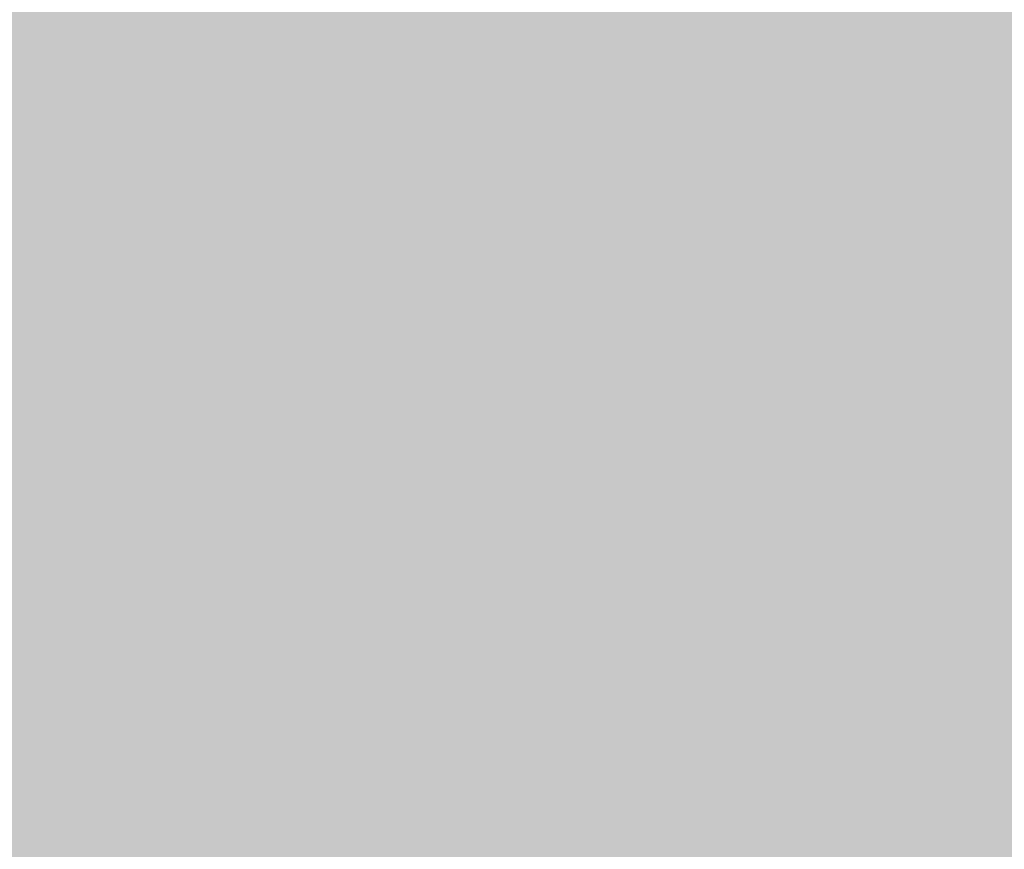
# Model space of a CAD drawing. Units: feet. Extents: x 3168 to 4724, y 827 to 1477.
# Tile 65 of 256: x 3273.15625 to 3273.17306, y 1099.00068 to 1099.01485. Entities that reach past the tile are written whole.
import ezdxf

# ---------------------------------------------------------------- set-up
doc = ezdxf.new("R2010")
doc.units = ezdxf.units.FT
doc.layers.add('A-ELEV', color=7, linetype='Continuous', lineweight=35)
doc.layers.add('A-ELEV-PATT', color=8, linetype='Continuous', lineweight=13)

msp = doc.modelspace()

# ---------------------------------------------------------------- hatches: boundary and pattern name
at = {"layer": 'A-ELEV-PATT'}
h = msp.add_hatch(color=256, dxfattribs=at)
h.dxf.hatch_style = 1
edge = h.paths.add_edge_path()
edge.add_ellipse((3552.905762, 979.220141), major_axis=(36.744924, 0), ratio=0.484848485, start_angle=0, end_angle=360)
edge = h.paths.add_edge_path()
edge.add_ellipse((3559.891637, 929.252282), major_axis=(36.744924, 0), ratio=0.484848485, start_angle=0, end_angle=360)
edge = h.paths.add_edge_path()
edge.add_line((3299.31681, 1198.606081), (3479.916714, 1198.606081))
edge.add_line((3479.916714, 1198.606081), (3479.916714, 1209.86857))
edge.add_spline(control_points=[(3479.916714, 1209.86857), (3464.301157, 1209.86857), (3448.685601, 1209.86857), (3410.949139, 1209.86857), (3388.828234, 1209.86857), (3355.646876, 1209.86857), (3344.586423, 1209.86857), (3327.995745, 1209.86857), (3322.465518, 1209.86857), (3314.170179, 1209.86857), (3311.405066, 1209.86857), (3307.257396, 1209.86857), (3305.874839, 1209.86857), (3303.801005, 1209.86857), (3303.109726, 1209.86857), (3302.072809, 1209.86857), (3301.72717, 1209.86857), (3301.208711, 1209.86857), (3301.035891, 1209.86857), (3300.776662, 1209.86857), (3300.690252, 1209.86857), (3300.560638, 1209.86857), (3300.517433, 1209.86857), (3300.452625, 1209.86857), (3300.431023, 1209.86857), (3300.398619, 1209.86857), (3300.387818, 1209.86857), (3300.366216, 1209.86857), (3300.345676, 1209.86857), (3300.345548, 1209.86857), (3300.345505, 1209.86857), (3300.343304, 1209.86857), (3300.341146, 1209.868571), (3300.337909, 1209.868571), (3300.33683, 1209.868572), (3300.333942, 1209.868573), (3300.332133, 1209.868574), (3300.325515, 1209.868577), (3300.320706, 1209.868581), (3300.310925, 1209.868592), (3300.305952, 1209.868598), (3300.290511, 1209.868623), (3300.280045, 1209.868646), (3300.232425, 1209.868777), (3300.195298, 1209.868954), (3299.951068, 1209.870608), (3299.744824, 1209.874326), (3299.436827, 1209.883257), (3299.334389, 1209.886792), (3299.181079, 1209.89292), (3299.130033, 1209.895099), (3298.652217, 1209.916801), (3298.22946, 1209.945718), (3297.601631, 1210.002367), (3297.393404, 1210.023464), (3297.082652, 1210.058309), (3296.979332, 1210.070458), (3296.292954, 1210.154861), (3295.718148, 1210.243356), (3294.868717, 1210.39885), (3294.5877, 1210.454478), (3294.169341, 1210.543349), (3294.030415, 1210.573878), (3291.707149, 1211.1012), (3289.65359, 1211.813435), (3285.776259, 1213.563988), (3283.95141, 1214.603478), (3280.512159, 1216.98008), (3278.897241, 1218.317592), (3276.379914, 1220.829489), (3275.416042, 1221.917738), (3274.039342, 1223.7077), (3273.581043, 1224.349535), (3273.143228, 1225.016316)], knot_values=[39.119033, 39.119033, 39.119033, 39.119033, 39.286353, 39.286353, 39.523379, 39.523379, 39.641892, 39.641892, 39.701148, 39.701148, 39.730777, 39.730777, 39.745591, 39.745591, 39.752998, 39.752998, 39.756701, 39.756701, 39.758553, 39.758553, 39.759479, 39.759479, 39.759942, 39.759942, 39.760173, 39.760173, 39.760289, 39.760289, 39.760405, 39.760405, 39.760463, 39.760463, 39.763389, 39.763389, 39.764851, 39.764851, 39.767304, 39.767304, 39.773825, 39.773825, 39.78057, 39.78057, 39.79477, 39.79477, 39.845194, 39.845194, 40.126715, 40.126715, 40.267476, 40.267476, 40.337856, 40.337856, 40.927023, 40.927023, 41.221606, 41.221606, 41.368898, 41.368898, 42.202622, 42.202622, 42.619485, 42.619485, 42.827916, 42.827916, 46.118323, 46.118323, 49.408731, 49.408731, 52.699139, 52.699139, 54.927489, 54.927489, 56.104228, 56.104228, 56.104228, 56.104228], weights=[1, 1, 1, 1, 1, 1, 1, 1, 1, 1, 1, 1, 1, 1, 1, 1, 1, 1, 1, 1, 1, 1, 1, 1, 1, 1, 1, 1, 1, 1, 1, 1, 1, 1, 1, 1, 1, 1, 1, 1, 1, 1, 1, 1, 1, 1, 1, 1, 1, 1, 1, 1, 1, 1, 1, 1, 1, 1, 1, 1, 1, 1, 1, 1, 1, 1, 1, 1, 1, 1, 1, 1, 1, 1], degree=3, periodic=0)
edge.add_line((3273.143228, 1225.016316), (3273.143228, 1099.016316))
edge.add_line((3273.143228, 1099.016316), (3299.31681, 1099.016316))
edge.add_line((3299.31681, 1099.016316), (3299.31681, 1198.606081))
edge = h.paths.add_edge_path()
edge.add_line((3304.758443, 1324.15806), (3479.916714, 1324.15806))
edge.add_line((3479.916714, 1324.15806), (3479.916714, 1335.714618))
edge.add_line((3479.916714, 1335.714618), (3269.161628, 1335.714618))
edge.add_spline(control_points=[(3269.161628, 1335.714618), (3264.024231, 1335.714618), (3258.364118, 1328.958189), (3259.264311, 1323.900274)], knot_values=[0, 0, 0, 0, 15.412191, 15.412191, 15.412191, 15.412191], degree=3, periodic=0)
edge.add_line((3259.264311, 1323.900274), (3265.516849, 1288.769135))
edge.add_line((3265.516849, 1288.769135), (3275.265103, 1261.545626))
edge.add_line((3275.265103, 1261.545626), (3304.758443, 1261.545626))
edge.add_line((3304.758443, 1261.545626), (3304.758443, 1324.15806))
h = msp.add_hatch(color=256, dxfattribs=at)
h.dxf.hatch_style = 1
h.paths.add_polyline_path([(3384.525247, 1099.016316), (3335.029168, 1099.016316), (3299.31681, 1099.016316), (3273.143228, 1099.016316), (3217.565364, 1099.016316), (3168.069285, 827.11626), (3335.029168, 827.11626)])

# ---------------------------------------------------------------- linework, layer by layer
at = {"layer": 'A-ELEV'}
msp.add_open_spline([(3808.5202, 1099.016316), (3808.5202, 1141.413235), (3808.5202, 1183.810154), (3808.5202, 1226.635324), (3808.5202, 1227.063576), (3808.5202, 1227.491828), (3811.491871, 1248.994673), (3814.463542, 1270.497518), (3817.46523, 1292.217564), (3817.495247, 1292.434764), (3817.525264, 1292.651964), (3817.572801, 1310.106748), (3817.620339, 1327.561532), (3817.667877, 1345.016316), (3817.667877, 1345.457962), (3817.667877, 1345.899608), (3817.667877, 1346.456047), (3817.667877, 1346.57084), (3817.667877, 1346.752887), (3817.667877, 1346.820142), (3817.667877, 1346.93487), (3817.667877, 1346.982345), (3817.667877, 1347.038587), (3817.667877, 1347.047356), (3817.667877, 1347.073661), (3817.667877, 1347.059303), (3817.667877, 1347.061545), (3817.667876, 1347.062667), (3817.667875, 1347.066031), (3817.667874, 1347.068274), (3817.66787, 1347.075001), (3817.667866, 1347.079486), (3817.667849, 1347.092937), (3817.667833, 1347.101902), (3817.667766, 1347.12879), (3817.667699, 1347.146705), (3817.667432, 1347.200421), (3817.667165, 1347.236192), (3817.6661, 1347.343385), (3817.665038, 1347.414686), (3817.660812, 1347.628095), (3817.656608, 1347.769708), (3817.63997, 1348.192487), (3817.623509, 1348.471586), (3817.559094, 1349.300067), (3817.496121, 1349.840588), (3817.255432, 1351.424156), (3817.026318, 1352.428785), (3816.306871, 1354.888914), (3815.743745, 1356.268727), (3814.463959, 1358.81921), (3813.746413, 1359.990968), (3812.195838, 1362.172343), (3811.362245, 1363.182124), (3809.588836, 1365.069009), (3808.648816, 1365.946105), (3806.654262, 1367.579616), (3805.599702, 1368.336154), (3803.352891, 1369.722327), (3802.160535, 1370.352386), (3799.600813, 1371.453586), (3798.232688, 1371.925481), (3795.280084, 1372.634624), (3793.693148, 1372.872068), (3791.869441, 1372.92648), (3791.740861, 1372.92922), (3791.353371, 1372.934101), (3791.092707, 1372.932901), (3790.304116, 1372.915068), (3789.769543, 1372.884195), (3789.20919, 1372.830236), (3789.190622, 1372.828424), (3789.134892, 1372.822912), (3789.097705, 1372.819137), (3789.048445, 1372.814008), (3789.0364, 1372.812743), (3789.000256, 1372.808918), (3788.976147, 1372.806325), (3788.949405, 1372.803404), (3788.946786, 1372.803118), (3788.942567, 1372.802655), (3788.940967, 1372.80248), (3788.938572, 1372.802217), (3788.937777, 1372.802129), (3788.935391, 1372.801867), (3788.867535, 1372.794402), (3788.756866, 1372.782228), (3788.701532, 1372.776141), (3788.53553, 1372.75788), (3788.424861, 1372.745707), (3788.092856, 1372.709185), (3787.871519, 1372.684837), (3787.207509, 1372.611793), (3786.764835, 1372.563097), (3785.436814, 1372.417009), (3784.551467, 1372.319617), (3781.895425, 1372.027442), (3780.12473, 1371.832658), (3774.812646, 1371.248307), (3771.271256, 1370.858739), (3760.647088, 1369.690037), (3753.56431, 1368.910902), (3732.315973, 1366.573498), (3718.150416, 1365.015228), (3694.006758, 1362.359326), (3684.028657, 1361.261694), (3674.050557, 1360.164062), (3664.600662, 1360.164062), (3655.150767, 1360.164062), (3626.801081, 1360.164062), (3607.901291, 1360.164062), (3551.20192, 1360.164062), (3513.40234, 1360.164062), (3467.725182, 1360.164062), (3459.847604, 1360.164062), (3436.214873, 1360.164062), (3420.459718, 1360.164062), (3373.194255, 1360.164062), (3341.683946, 1360.164062), (3302.848162, 1360.164062), (3295.522686, 1360.164062), (3286.038292, 1360.164062), (3283.879372, 1360.164062), (3277.402613, 1360.164062), (3273.084773, 1360.164062), (3267.732851, 1360.164062), (3266.698768, 1360.164062), (3263.59652, 1360.164062), (3261.528355, 1360.164062), (3259.236943, 1360.164062), (3259.013697, 1360.164062), (3258.343958, 1360.164062), (3257.897466, 1360.164062), (3257.430998, 1360.164062), (3257.411022, 1360.164062), (3257.370573, 1360.164062), (3257.37547, 1360.164062), (3257.374598, 1360.164062), (3257.373937, 1360.164062), (3257.371956, 1360.164062), (3257.370635, 1360.164061), (3257.366673, 1360.16406), (3257.364032, 1360.164059), (3257.356109, 1360.164053), (3257.350828, 1360.164047), (3257.334987, 1360.164023), (3257.32443, 1360.163998), (3257.292769, 1360.163899), (3257.271676, 1360.163799), (3257.208439, 1360.163398), (3257.166337, 1360.162995), (3257.040206, 1360.161388), (3256.956349, 1360.159783), (3256.705504, 1360.153393), (3256.53924, 1360.147036), (3256.04357, 1360.121916), (3255.717296, 1360.097102), (3254.752446, 1360.000481), (3254.127968, 1359.906513), (3252.180067, 1359.525332), (3250.941574, 1359.143991), (3248.670175, 1358.24329), (3247.635739, 1357.723834), (3245.732632, 1356.603471), (3244.863388, 1356.00206), (3243.253108, 1354.742865), (3242.511972, 1354.084731), (3240.751052, 1352.344781), (3239.800961, 1351.229574), (3238.087769, 1348.87244), (3237.324685, 1347.630355), (3235.98251, 1344.971632), (3235.402205, 1343.554907), (3234.591081, 1340.815458), (3234.310882, 1339.54355), (3233.97649, 1336.802561), (3233.922113, 1335.330877), (3234.148916, 1332.591269), (3234.349529, 1331.367201), (3234.719893, 1329.999367), (3234.752423, 1329.883362), (3234.853619, 1329.534797), (3234.925892, 1329.301685), (3235.024836, 1329.002552), (3235.046924, 1328.936928), (3235.077639, 1328.847239), (3235.085924, 1328.823198), (3235.110939, 1328.751064), (3235.127828, 1328.702962), (3235.147992, 1328.646242), (3235.151059, 1328.637632), (3235.156096, 1328.623526), (3235.158061, 1328.61803), (3235.160209, 1328.61203), (3235.165612, 1328.596943), (3235.180099, 1328.556486), (3235.190263, 1328.528101), (3235.220756, 1328.442946), (3235.241084, 1328.386176), (3235.302069, 1328.215865), (3235.342726, 1328.102325), (3235.464696, 1327.761704), (3235.54601, 1327.534623), (3235.78995, 1326.853381), (3235.952577, 1326.39922), (3236.440459, 1325.036736), (3236.765713, 1324.128414), (3237.741475, 1321.403446), (3238.391983, 1319.586801), (3240.343508, 1314.136866), (3241.644525, 1310.503576), (3245.547574, 1299.603706), (3248.149607, 1292.337126), (3255.955706, 1270.537385), (3261.159772, 1256.004225), (3267.387618, 1238.612001), (3268.411397, 1235.752937), (3269.510378, 1232.683864), (3269.585579, 1232.473854), (3269.706612, 1232.135851), (3269.752444, 1232.007857), (3269.827329, 1231.79873), (3269.856382, 1231.717595), (3269.906325, 1231.578122), (3269.927215, 1231.519782), (3269.972468, 1231.393406), (3269.996831, 1231.325368), (3270.026503, 1231.242506), (3270.031811, 1231.227681), (3270.040282, 1231.204024), (3270.039224, 1231.206979), (3270.039359, 1231.206601), (3270.039427, 1231.206412), (3270.03963, 1231.205846), (3270.039765, 1231.205468), (3270.040171, 1231.204335), (3270.040442, 1231.203579), (3270.041254, 1231.201313), (3270.041796, 1231.199802), (3270.04342, 1231.195269), (3270.044504, 1231.192248), (3270.047756, 1231.183185), (3270.049926, 1231.177145), (3270.056442, 1231.159028), (3270.060793, 1231.146957), (3270.073867, 1231.110761), (3270.082613, 1231.086656), (3270.108936, 1231.014413), (3270.1266, 1230.96635), (3270.179934, 1230.822457), (3270.215947, 1230.726923), (3270.325323, 1230.441508), (3270.400026, 1230.252811), (3270.629249, 1229.691444), (3270.788883, 1229.323501), (3271.286488, 1228.238319), (3271.6431, 1227.539755), (3272.775859, 1225.515277), (3273.614169, 1224.260502), (3275.416042, 1221.917738), (3276.379914, 1220.829489), (3278.897241, 1218.317592), (3280.512159, 1216.98008), (3283.95141, 1214.603478), (3285.776259, 1213.563988), (3289.65359, 1211.813435), (3291.707149, 1211.1012), (3294.030415, 1210.573878), (3294.169341, 1210.543349), (3294.5877, 1210.454478), (3294.868717, 1210.39885), (3295.718148, 1210.243356), (3296.292954, 1210.154861), (3296.979332, 1210.070458), (3297.082652, 1210.058309), (3297.393404, 1210.023464), (3297.601631, 1210.002367), (3298.22946, 1209.945718), (3298.652217, 1209.916801), (3299.130033, 1209.895099), (3299.181079, 1209.89292), (3299.334389, 1209.886792), (3299.436827, 1209.883257), (3299.744824, 1209.874326), (3299.951068, 1209.870608), (3300.195298, 1209.868954), (3300.232425, 1209.868777), (3300.280045, 1209.868646), (3300.290511, 1209.868623), (3300.305952, 1209.868598), (3300.310925, 1209.868592), (3300.320706, 1209.868581), (3300.325515, 1209.868577), (3300.332133, 1209.868574), (3300.333942, 1209.868573), (3300.33683, 1209.868572), (3300.337909, 1209.868571), (3300.341146, 1209.868571), (3300.343304, 1209.86857), (3300.345505, 1209.86857), (3300.345548, 1209.86857), (3300.345676, 1209.86857), (3300.366216, 1209.86857), (3300.387818, 1209.86857), (3300.398619, 1209.86857), (3300.431023, 1209.86857), (3300.452625, 1209.86857), (3300.517433, 1209.86857), (3300.560638, 1209.86857), (3300.690252, 1209.86857), (3300.776662, 1209.86857), (3301.035891, 1209.86857), (3301.208711, 1209.86857), (3301.72717, 1209.86857), (3302.072809, 1209.86857), (3303.109726, 1209.86857), (3303.801005, 1209.86857), (3305.874839, 1209.86857), (3307.257396, 1209.86857), (3311.405066, 1209.86857), (3314.170179, 1209.86857), (3322.465518, 1209.86857), (3327.995745, 1209.86857), (3344.586423, 1209.86857), (3355.646876, 1209.86857), (3388.828234, 1209.86857), (3410.949139, 1209.86857), (3477.311855, 1209.86857), (3521.553665, 1209.86857), (3566.836184, 1209.86857), (3567.876892, 1209.86857), (3570.999017, 1209.86857), (3573.080433, 1209.86857), (3575.781396, 1209.86857), (3576.400943, 1209.86857), (3577.295821, 1209.86857), (3577.571152, 1209.86857), (3578.397146, 1209.86857), (3578.947808, 1209.86857), (3579.756491, 1209.86857), (3580.014511, 1209.86857), (3580.342737, 1209.86857), (3580.326865, 1209.86857), (3580.32717, 1209.86857), (3580.327323, 1209.86857), (3580.327781, 1209.86857), (3580.328086, 1209.86857), (3580.329002, 1209.86857), (3580.329613, 1209.86857), (3580.331445, 1209.86857), (3580.332667, 1209.86857), (3580.336332, 1209.868569), (3580.338775, 1209.868567), (3580.346107, 1209.868563), (3580.350995, 1209.868558), (3580.365663, 1209.86854), (3580.375445, 1209.868522), (3580.404801, 1209.868449), (3580.424386, 1209.868376), (3580.483183, 1209.868085), (3580.522437, 1209.867793), (3580.640361, 1209.866624), (3580.719195, 1209.865454), (3580.956315, 1209.860766), (3581.115222, 1209.85607), (3581.594164, 1209.83723), (3581.916419, 1209.818331), (3582.889947, 1209.742428), (3583.547986, 1209.666169), (3585.531827, 1209.360617), (3586.867216, 1209.053886), (3589.471545, 1208.252472), (3590.740241, 1207.757852), (3591.995451, 1207.158802), (3592.057809, 1207.12874), (3592.244242, 1207.037954), (3592.367676, 1206.976632), (3592.73528, 1206.790359), (3592.976752, 1206.663101), (3593.244539, 1206.516441), (3593.274731, 1206.499825), (3593.365115, 1206.449839), (3593.425113, 1206.416333), (3593.604314, 1206.315285), (3593.722725, 1206.247211), (3593.857212, 1206.168398), (3593.874362, 1206.158319), (3593.925741, 1206.128041), (3593.959899, 1206.107798), (3594.062086, 1206.046899), (3594.129827, 1206.006074), (3594.208436, 1205.958171), (3594.219683, 1205.951304), (3594.253391, 1205.930686), (3594.275819, 1205.916917), (3594.342972, 1205.875536), (3594.387563, 1205.847853), (3594.433616, 1205.81905), (3594.435256, 1205.818024), (3594.440175, 1205.814946), (3594.443453, 1205.812894), (3594.447123, 1205.810594), (3594.447516, 1205.810348), (3594.448695, 1205.80961), (3594.449481, 1205.809117), (3594.450366, 1205.808562), (3594.450466, 1205.8085), (3594.4506, 1205.808415), (3594.467399, 1205.797887), (3594.493269, 1205.781674), (3594.506204, 1205.773568), (3594.545008, 1205.749248), (3594.570878, 1205.733035), (3594.648487, 1205.684396), (3594.700226, 1205.651969), (3594.855444, 1205.554691), (3594.958922, 1205.489839), (3595.269357, 1205.295282), (3595.476314, 1205.165577), (3596.097185, 1204.776463), (3596.511099, 1204.517054), (3597.752841, 1203.738826), (3598.580669, 1203.220007), (3601.064152, 1201.663551), (3602.719807, 1200.625914), (3607.686774, 1197.513002), (3610.998085, 1195.437727), (3620.932018, 1189.211903), (3627.55464, 1185.061354), (3647.422507, 1172.609707), (3660.667751, 1164.308608), (3700.403484, 1139.405313), (3726.893973, 1122.803116), (3757.205715, 1103.806052), (3761.02697, 1101.411184), (3764.848224, 1099.016316), (3745.328271, 1099.016316), (3725.808319, 1099.016316), (3706.288366, 1099.016316), (3706.288366, 1108.453237), (3706.288366, 1117.890158), (3706.288366, 1127.327079), (3710.750754, 1127.327079), (3715.213143, 1127.327079), (3719.675531, 1127.327079)], degree=3, knots=[0, 0, 0, 0, 0.982037, 0.982037, 0.991957, 0.991957, 0.991957, 1.966522, 1.966522, 1.976367, 1.976367, 1.976367, 2.976367, 2.976367, 2.976367, 3.00169, 3.00169, 3.008272, 3.008272, 3.012129, 3.012129, 3.014851, 3.014851, 3.015353, 3.015353, 3.016359, 3.016359, 3.017365, 3.017365, 3.019376, 3.019376, 3.023398, 3.023398, 3.031442, 3.031442, 3.047531, 3.047531, 3.079708, 3.079708, 3.144063, 3.144063, 3.272772, 3.272772, 3.53019, 3.53019, 4.045026, 4.045026, 5.074698, 5.074698, 6.700878, 6.700878, 8.327058, 8.327058, 9.953238, 9.953238, 11.579418, 11.579418, 13.205598, 13.205598, 14.831778, 14.831778, 16.457958, 16.457958, 18.084138, 18.084138, 18.206872, 18.206872, 18.45234, 18.45234, 18.943275, 18.943275, 18.960093, 18.960093, 18.993729, 18.993729, 19.00461, 19.00461, 19.026374, 19.026374, 19.028737, 19.028737, 19.03018, 19.03018, 19.030897, 19.030897, 19.032332, 19.032332, 19.033766, 19.033766, 19.036636, 19.036636, 19.042374, 19.042374, 19.053851, 19.053851, 19.076805, 19.076805, 19.122714, 19.122714, 19.21453, 19.21453, 19.398163, 19.398163, 19.765429, 19.765429, 20.024128, 20.024128, 20.024128, 20.092031, 20.092031, 20.227836, 20.227836, 20.499446, 20.499446, 20.556051, 20.556051, 20.66926, 20.66926, 20.895678, 20.895678, 20.948316, 20.948316, 20.963829, 20.963829, 20.994855, 20.994855, 21.002285, 21.002285, 21.017146, 21.017146, 21.01875, 21.01875, 21.021959, 21.021959, 21.022102, 21.022102, 21.022249, 21.022249, 21.022708, 21.022708, 21.023627, 21.023627, 21.025464, 21.025464, 21.029138, 21.029138, 21.036486, 21.036486, 21.051183, 21.051183, 21.080575, 21.080575, 21.139361, 21.139361, 21.256932, 21.256932, 21.492073, 21.492073, 21.962356, 21.962356, 23.01002, 23.01002, 24.057684, 24.057684, 25.105348, 25.105348, 26.153011, 26.153011, 27.776787, 27.776787, 29.400562, 29.400562, 31.024337, 31.024337, 32.278801, 32.278801, 33.533265, 33.533265, 34.467568, 34.467568, 34.553971, 34.553971, 34.726776, 34.726776, 34.775309, 34.775309, 34.793079, 34.793079, 34.82862, 34.82862, 34.834979, 34.834979, 34.839039, 34.839039, 34.839411, 34.839411, 34.840285, 34.840285, 34.842034, 34.842034, 34.845531, 34.845531, 34.852525, 34.852525, 34.866512, 34.866512, 34.894488, 34.894488, 34.950439, 34.950439, 35.062342, 35.062342, 35.286147, 35.286147, 35.733758, 35.733758, 35.821815, 35.821815, 35.828283, 35.828283, 35.832225, 35.832225, 35.834724, 35.834724, 35.836521, 35.836521, 35.838617, 35.838617, 35.839073, 35.839073, 35.839345, 35.839345, 35.839617, 35.839617, 35.840161, 35.840161, 35.841249, 35.841249, 35.843425, 35.843425, 35.847778, 35.847778, 35.856482, 35.856482, 35.873891, 35.873891, 35.908709, 35.908709, 35.978345, 35.978345, 36.117617, 36.117617, 36.396161, 36.396161, 36.953248, 36.953248, 38.067423, 38.067423, 40.295772, 40.295772, 42.524122, 42.524122, 45.81453, 45.81453, 49.104937, 49.104937, 52.395345, 52.395345, 52.603776, 52.603776, 53.020639, 53.020639, 53.854363, 53.854363, 54.001655, 54.001655, 54.296238, 54.296238, 54.885405, 54.885405, 54.955785, 54.955785, 55.096546, 55.096546, 55.378067, 55.378067, 55.42849, 55.42849, 55.442691, 55.442691, 55.449436, 55.449436, 55.455957, 55.455957, 55.458409, 55.458409, 55.459872, 55.459872, 55.462798, 55.462798, 55.462856, 55.462856, 55.462972, 55.462972, 55.463088, 55.463088, 55.463319, 55.463319, 55.463782, 55.463782, 55.464708, 55.464708, 55.46656, 55.46656, 55.470263, 55.470263, 55.47767, 55.47767, 55.492484, 55.492484, 55.522112, 55.522112, 55.581369, 55.581369, 55.699882, 55.699882, 55.936907, 55.936907, 56.410959, 56.410959, 56.42211, 56.42211, 56.444413, 56.444413, 56.451051, 56.451051, 56.454001, 56.454001, 56.459901, 56.459901, 56.462666, 56.462666, 56.463418, 56.463418, 56.464171, 56.464171, 56.465675, 56.465675, 56.468684, 56.468684, 56.474702, 56.474702, 56.486738, 56.486738, 56.51081, 56.51081, 56.558955, 56.558955, 56.655243, 56.655243, 56.847821, 56.847821, 57.232975, 57.232975, 58.003284, 58.003284, 59.543901, 59.543901, 62.625137, 62.625137, 68.787607, 68.787607, 74.950078, 74.950078, 75.27336, 75.27336, 75.919923, 75.919923, 77.213051, 77.213051, 77.377769, 77.377769, 77.707206, 77.707206, 78.366079, 78.366079, 78.462532, 78.462532, 78.655436, 78.655436, 79.041245, 79.041245, 79.105735, 79.105735, 79.234714, 79.234714, 79.492672, 79.492672, 79.502197, 79.502197, 79.521249, 79.521249, 79.523534, 79.523534, 79.528103, 79.528103, 79.528682, 79.528682, 79.528885, 79.528885, 79.529089, 79.529089, 79.529495, 79.529495, 79.530308, 79.530308, 79.531935, 79.531935, 79.535187, 79.535187, 79.541693, 79.541693, 79.554704, 79.554704, 79.580725, 79.580725, 79.632769, 79.632769, 79.736856, 79.736856, 79.94503, 79.94503, 80.361377, 80.361377, 80.421435, 80.421435, 80.421435, 81.421435, 81.421435, 81.421435, 82.421435, 82.421435, 82.421435, 83.421435, 83.421435, 83.421435, 83.421435], dxfattribs=at)

doc.saveas('drawing.dxf')
